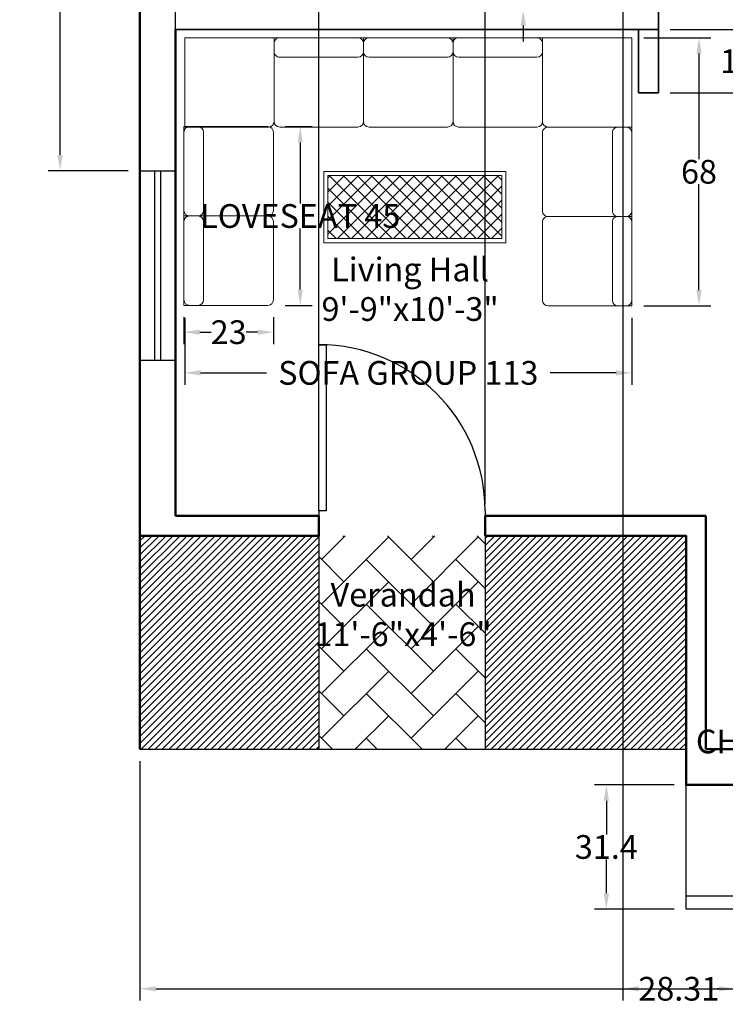
# Model space of a CAD drawing. Units: inches. Extents: x 89 to 490, y -59 to 378.
# Tile 1 of 20: x 97 to 275, y -51 to 198. Entities that reach past the tile are written whole.
import ezdxf

# ---------------------------------------------------------------- set-up
doc = ezdxf.new("R2010")
doc.units = ezdxf.units.IN
doc.header["$MEASUREMENT"] = 0
for name, color, linetype, lineweight in [('A-ANNO-DIMS', 2, 'Continuous', 18), ('A-AREA-IDEN', 7, 'Continuous', 18), ('A-FLOR-PATT', 3, 'Continuous', 13), ('A-FURN-PATT', 55, 'Continuous', 13), ('Center Table', 54, 'Continuous', 18), ('Doors', 34, 'Continuous', 25), ('Inner Walls', 31, 'Continuous', 35), ('L-PLNT-EDGE', 31, 'Continuous', 25), ('Outer Walls', 12, 'Continuous', 50), ('Sofa', 114, 'Continuous', 18), ('Verandah', 3, 'Continuous', 25), ('Windows', 171, 'Continuous', 25)]:
    doc.layers.add(name, color=color, linetype=linetype, lineweight=lineweight)
doc.styles.get("Standard").update_dxf_attribs({"font": 'arial.ttf'})
doc.dimstyles.get("Standard").update_dxf_attribs({"dimtxt": 6, "dimasz": 4, "dimexe": 3, "dimexo": 3, "dimgap": 0.09, "dimtad": 0, "dimtih": 1, "dimtoh": 1, "dimdec": 1, "dimzin": 0, "dimdsep": 46, "dimlunit": 3, "dimtxsty": 'Standard', "dimcen": 0.09, "dimadec": 0, "dimazin": 0, "dimtfac": 1, "dimtdec": 1, "dimtofl": 0, "dimtmove": 0, "dimatfit": 3, "dimfxl": 1, "dimtolj": 1, "dimtzin": 0, "dimarcsym": 0})

# ---------------------------------------------------------------- blocks, each defined once
blk = doc.blocks.new('*U6')
for p, q in [((0, 0), (0, -6)), ((40, 0), (40, -6))]:
    blk.add_line(p, q)
blk.add_lwpolyline([(0, 0), (0, 40), (1.75, 40), (1.75, 0)], close=True)
blk.add_arc((0, 0), 40, 0, 90)
blk = doc.blocks.new('A$C51FB459E')
for p, q in [((0, 1.6), (0, 2.4)), ((0, 2.4), (0.75, 2.4)), ((0.05, 2.4), (0.125, 2.4)), ((0, 1.65), (0, 2.35)), ((0.175, 2.35), (0.175, 1.65)), ((0.8, 2.35), (0.8, 1.65)), ((0, 0.8), (0, 1.6)), ((0, 1.6), (0.75, 1.6)), ((0.75, 1.6), (0, 1.6)), ((0.05, 1.6), (0.125, 1.6)), ((0.125, 1.6), (0.05, 1.6)), ((0, 0.85), (0, 1.55)), ((0.175, 1.55), (0.175, 0.85)), ((0.8, 1.55), (0.8, 0.85)), ((0, 0), (0, 0.8)), ((0, 0.8), (0.75, 0.8)), ((0.75, 0.8), (0, 0.8)), ((0.125, 0.8), (0.05, 0.8)), ((0.85, 0.8), (1.55, 0.8)), ((1.65, 0.8), (2.35, 0.8)), ((2.45, 0.8), (3.15, 0.8)), ((3.9996, 0.8), (3.25, 0.8)), ((3.9996, 0), (3.9996, 0.8)), ((0.8, 0), (0.8, 0.75)), ((0.8, 0.75), (0.8, 0)), ((1.6, 0), (1.6, 0.75)), ((1.6, 0.75), (1.6, 0)), ((2.4, 0.75), (2.4, 0)), ((2.4, 0), (2.4, 0.75)), ((3.2, 0.75), (3.2, 0)), ((3.2, 0.75), (3.2, 0)), ((0.8, 0.05), (0.8, 0.125)), ((0.85, 0.175), (1.55, 0.175)), ((1.6, 0.05), (1.6, 0.125)), ((1.6, 0.125), (1.6, 0.05)), ((1.65, 0.175), (2.35, 0.175)), ((2.4, 0.125), (2.4, 0.05)), ((2.4, 0.05), (2.4, 0.125)), ((2.45, 0.175), (3.15, 0.175)), ((3.2, 0.125), (3.2, 0.05)), ((0.8, 0), (0, 0)), ((1.6, 0), (0.8, 0)), ((1.55, 0), (0.85, 0)), ((2.4, 0), (1.6, 0)), ((2.35, 0), (1.65, 0)), ((3.2, 0), (2.4, 0)), ((3.15, 0), (2.45, 0)), ((3.2, 0), (3.9996, 0))]:
    blk.add_line(p, q)
for centre, start, end in [((0.05, 2.35), 90, 180), ((0.125, 2.35), 0, 90), ((0.75, 2.35), 0, 90), ((0.05, 1.65), 180, 270), ((0.05, 1.55), 90, 180), ((0.125, 1.65), 270, 0), ((0.125, 1.55), 360, 90), ((0.75, 1.65), 270, 0), ((0.75, 1.55), 360, 90), ((0.05, 0.85), 180, 270), ((0.125, 0.85), 270, 0), ((0.75, 0.85), 270, 0), ((0.75, 0.75), 0, 90), ((0.85, 0.75), 90, 180), ((1.55, 0.75), 0, 90), ((1.65, 0.75), 90, 180), ((2.35, 0.75), 0, 90), ((2.45, 0.75), 90, 180), ((3.15, 0.75), 0, 90), ((3.25, 0.75), 90, 180), ((0.85, 0.125), 90, 180), ((1.55, 0.125), 0, 90), ((1.65, 0.125), 90, 180), ((2.35, 0.125), 0, 90), ((2.45, 0.125), 90, 180), ((3.15, 0.125), 360, 90), ((0.85, 0.05), 180, 270), ((1.55, 0.05), 270, 0), ((1.65, 0.05), 180, 270), ((2.35, 0.05), 270, 360), ((2.45, 0.05), 180, 270), ((3.15, 0.05), 270, 0)]:
    blk.add_arc(centre, 0.05, start, end)
blk = doc.blocks.new('small sofa')
for p, q in [((881.35, 152.51), (860.16, 152.51)), ((860.16, 152.51), (881.35, 152.51)), ((877.82, 152.51), (879.94, 152.51)), ((881.35, 152.51), (881.35, 129.91)), ((858.75, 131.32), (858.75, 151.1)), ((876.41, 131.32), (876.41, 151.1)), ((881.35, 151.1), (881.35, 131.32)), ((881.35, 129.91), (860.16, 129.91)), ((860.16, 129.91), (881.35, 129.91)), ((879.94, 129.91), (877.82, 129.91)), ((877.82, 129.91), (879.94, 129.91)), ((881.35, 129.91), (881.35, 107.31)), ((858.75, 108.72), (858.75, 128.5)), ((876.41, 108.72), (876.41, 128.5)), ((881.35, 128.5), (881.35, 108.72)), ((881.35, 107.31), (860.16, 107.31)), ((879.94, 107.31), (877.82, 107.31))]:
    blk.add_line(p, q)
for centre, start, end in [((860.16, 151.1), 90, 180), ((877.82, 151.1), 90, 180), ((879.94, 151.1), 0, 90), ((860.16, 131.32), 180, 270), ((860.16, 128.5), 90, 180), ((877.82, 131.32), 180, 270), ((877.82, 128.5), 90, 180), ((879.94, 131.32), 270, 0), ((879.94, 128.5), 0, 90), ((860.16, 108.72), 180, 270), ((877.82, 108.72), 180, 270), ((879.94, 108.72), 270, 0)]:
    blk.add_arc(centre, 1.41, start, end)
blk = doc.blocks.new('WIN-48x9')
for p, q in [((3.8, 0), (3.8, 48)), ((5.2, 48), (5.2, 0))]:
    blk.add_line(p, q)
blk.add_lwpolyline([(9, 0), (0, 0), (0, 48), (9, 48)], close=True)
blk = doc.blocks.new('*D28')
at = {"layer": 'A-ANNO-DIMS', "color": 0, "lineweight": -2, "transparency": 16777216}
for p, q in [((326.43, 33.4), (324.38, 33.4)), ((327.38, 29.4), (327.38, 23.72)), ((326.43, 19.72), (324.38, 19.72)), ((327.38, 19.72), (327.38, 15.72)), ((327.38, 15.72), (323.38, 15.72))]:
    blk.add_line(p, q, dxfattribs=at)
at = {"layer": 'A-ANNO-DIMS', "color": 0, "transparency": 16777216}
for points in [[(326.71, 29.4), (328.05, 29.4), (327.38, 33.4)], [(326.71, 23.72), (328.05, 23.72), (327.38, 19.72)]]:
    blk.add_solid(points, dxfattribs=at)
at = {"layer": 'Defpoints', "color": 0, "transparency": 16777216}
for p in [(329.43, 33.4), (327.38, 19.72), (329.43, 19.72)]:
    blk.add_point(p, dxfattribs=at)
at = {"layer": 'A-ANNO-DIMS', "color": 0, "transparency": 16777216, "insert": (294.52, 15.72), "char_height": 6, "attachment_point": 5}
blk.add_mtext('\\A1;CHAIR 14 TYP.', dxfattribs=at)
blk = doc.blocks.new('*D38')
at = {"layer": 'A-ANNO-DIMS', "color": 0, "lineweight": -2, "transparency": 16777216}
for p, q in [((138.75, 122.88), (138.75, 105.93)), ((251.75, 122.88), (251.75, 105.93)), ((142.75, 108.93), (159.44, 108.93)), ((247.75, 108.93), (231.06, 108.93))]:
    blk.add_line(p, q, dxfattribs=at)
at = {"layer": 'A-ANNO-DIMS', "color": 0, "transparency": 16777216}
for points in [[(142.75, 109.59), (142.75, 108.26), (138.75, 108.93)], [(247.75, 109.59), (247.75, 108.26), (251.75, 108.93)]]:
    blk.add_solid(points, dxfattribs=at)
at = {"layer": 'Defpoints', "color": 0, "transparency": 16777216}
for p in [(138.75, 125.88), (251.75, 125.88), (138.75, 108.93)]:
    blk.add_point(p, dxfattribs=at)
at = {"layer": 'A-ANNO-DIMS', "color": 0, "transparency": 16777216, "insert": (195.25, 108.93), "char_height": 6, "attachment_point": 5}
blk.add_mtext('\\A1;SOFA GROUP 113', dxfattribs=at)
blk = doc.blocks.new('*D39')
at = {"layer": 'A-ANNO-DIMS', "color": 0, "lineweight": -2, "transparency": 16777216}
for p, q in [((254.75, 193.68), (271.7, 193.68)), ((268.7, 189.68), (268.7, 162.93)), ((268.7, 129.88), (268.7, 156.63)), ((254.75, 125.88), (271.7, 125.88))]:
    blk.add_line(p, q, dxfattribs=at)
at = {"layer": 'A-ANNO-DIMS', "color": 0, "transparency": 16777216}
for points in [[(268.04, 189.68), (269.37, 189.68), (268.7, 193.68)], [(268.04, 129.88), (269.37, 129.88), (268.7, 125.88)]]:
    blk.add_solid(points, dxfattribs=at)
at = {"layer": 'Defpoints', "color": 0, "transparency": 16777216}
for p in [(251.75, 193.68), (251.75, 125.88), (268.7, 125.88)]:
    blk.add_point(p, dxfattribs=at)
at = {"layer": 'A-ANNO-DIMS', "color": 0, "transparency": 16777216, "insert": (268.7, 159.78), "char_height": 6, "attachment_point": 5}
blk.add_mtext('\\A1;68', dxfattribs=at)
blk = doc.blocks.new('*D40')
at = {"layer": 'A-ANNO-DIMS', "color": 0, "lineweight": -2, "transparency": 16777216}
for p, q in [((164.17, 171.2), (170.95, 171.2)), ((167.95, 167.2), (167.95, 151.8)), ((167.95, 130), (167.95, 145.41)), ((164.17, 126), (170.95, 126))]:
    blk.add_line(p, q, dxfattribs=at)
at = {"layer": 'A-ANNO-DIMS', "color": 0, "transparency": 16777216}
for points in [[(167.29, 167.2), (168.62, 167.2), (167.95, 171.2)], [(167.29, 130), (168.62, 130), (167.95, 126)]]:
    blk.add_solid(points, dxfattribs=at)
at = {"layer": 'Defpoints', "color": 0, "transparency": 16777216}
for p in [(161.17, 171.2), (161.17, 126), (167.95, 126)]:
    blk.add_point(p, dxfattribs=at)
at = {"layer": 'A-ANNO-DIMS', "color": 0, "transparency": 16777216, "insert": (167.95, 148.6), "char_height": 6, "attachment_point": 5}
blk.add_mtext('\\A1;LOVESEAT 45', dxfattribs=at)
blk = doc.blocks.new('*D41')
at = {"layer": 'A-ANNO-DIMS', "color": 0, "lineweight": -2, "transparency": 16777216}
for p, q in [((138.57, 123), (138.57, 116.22)), ((161.17, 123), (161.17, 116.22)), ((142.57, 119.22), (145.43, 119.22)), ((157.17, 119.22), (154.31, 119.22))]:
    blk.add_line(p, q, dxfattribs=at)
at = {"layer": 'A-ANNO-DIMS', "color": 0, "transparency": 16777216}
for points in [[(142.57, 119.89), (142.57, 118.55), (138.57, 119.22)], [(157.17, 119.89), (157.17, 118.55), (161.17, 119.22)]]:
    blk.add_solid(points, dxfattribs=at)
at = {"layer": 'Defpoints', "color": 0, "transparency": 16777216}
for p in [(138.57, 126), (161.17, 126), (138.57, 119.22)]:
    blk.add_point(p, dxfattribs=at)
at = {"layer": 'A-ANNO-DIMS', "color": 0, "transparency": 16777216, "insert": (149.87, 119.22), "char_height": 6, "attachment_point": 5}
blk.add_mtext('\\A1;23', dxfattribs=at)
blk = doc.blocks.new('*D48')
at = {"layer": 'A-ANNO-DIMS', "color": 0, "lineweight": -2, "transparency": 16777216}
for p, q in [((127.44, 10.74), (127.44, -49.81)), ((459.44, -29.66), (459.44, -49.81)), ((131.44, -46.81), (286.76, -46.81)), ((455.44, -46.81), (300.13, -46.81))]:
    blk.add_line(p, q, dxfattribs=at)
at = {"layer": 'A-ANNO-DIMS', "color": 0, "transparency": 16777216}
for points in [[(131.44, -46.14), (131.44, -47.48), (127.44, -46.81)], [(455.44, -46.14), (455.44, -47.48), (459.44, -46.81)]]:
    blk.add_solid(points, dxfattribs=at)
at = {"layer": 'Defpoints', "color": 0, "transparency": 16777216}
for p in [(127.44, 13.74), (459.44, -26.66), (459.44, -46.81)]:
    blk.add_point(p, dxfattribs=at)
at = {"layer": 'A-ANNO-DIMS', "color": 0, "transparency": 16777216, "insert": (293.44, -46.81), "char_height": 6, "attachment_point": 5}
blk.add_mtext('\\A1;332', dxfattribs=at)
blk = doc.blocks.new('*D50')
at = {"layer": 'A-ANNO-DIMS', "color": 0, "lineweight": -2, "transparency": 16777216}
for p, q in [((262.44, 4.74), (242.29, 4.74)), ((245.29, 0.74), (245.29, -7.8)), ((245.29, -22.66), (245.29, -14.11)), ((262.44, -26.66), (242.29, -26.66))]:
    blk.add_line(p, q, dxfattribs=at)
at = {"layer": 'A-ANNO-DIMS', "color": 0, "transparency": 16777216}
for points in [[(244.62, 0.74), (245.96, 0.74), (245.29, 4.74)], [(244.62, -22.66), (245.96, -22.66), (245.29, -26.66)]]:
    blk.add_solid(points, dxfattribs=at)
at = {"layer": 'Defpoints', "color": 0, "transparency": 16777216}
for p in [(245.29, 4.74), (265.44, 4.74), (265.44, -26.66)]:
    blk.add_point(p, dxfattribs=at)
at = {"layer": 'A-ANNO-DIMS', "color": 0, "transparency": 16777216, "insert": (245.29, -10.96), "char_height": 6, "attachment_point": 5}
blk.add_mtext('\\A1;31.4', dxfattribs=at)
blk = doc.blocks.new('*D52')
at = {"layer": 'A-ANNO-DIMS', "color": 0, "lineweight": -2, "transparency": 16777216}
for p, q in [((124.44, 253.3), (104.29, 253.3)), ((107.29, 249.3), (107.29, 209.83)), ((107.29, 164.06), (107.29, 203.52)), ((124.44, 160.06), (104.29, 160.06))]:
    blk.add_line(p, q, dxfattribs=at)
at = {"layer": 'A-ANNO-DIMS', "color": 0, "transparency": 16777216}
for points in [[(106.62, 249.3), (107.96, 249.3), (107.29, 253.3)], [(106.62, 164.06), (107.96, 164.06), (107.29, 160.06)]]:
    blk.add_solid(points, dxfattribs=at)
at = {"layer": 'Defpoints', "color": 0, "transparency": 16777216}
for p in [(127.44, 253.3), (107.29, 160.06), (127.44, 160.06)]:
    blk.add_point(p, dxfattribs=at)
at = {"layer": 'A-ANNO-DIMS', "color": 0, "transparency": 16777216, "insert": (107.29, 206.68), "char_height": 6, "attachment_point": 5}
blk.add_mtext('\\A1;93.25', dxfattribs=at)
blk = doc.blocks.new('*D57')
at = {"layer": 'A-ANNO-DIMS', "color": 0, "lineweight": -2, "transparency": 16777216}
for p, q in [((172.65, 75.74), (172.65, 376.89)), ((214.65, 75.74), (214.65, 376.89)), ((176.65, 373.89), (189.17, 373.89)), ((210.65, 373.89), (198.13, 373.89))]:
    blk.add_line(p, q, dxfattribs=at)
at = {"layer": 'A-ANNO-DIMS', "color": 0, "transparency": 16777216}
for points in [[(176.65, 374.56), (176.65, 373.22), (172.65, 373.89)], [(210.65, 374.56), (210.65, 373.22), (214.65, 373.89)]]:
    blk.add_solid(points, dxfattribs=at)
at = {"layer": 'Defpoints', "color": 0, "transparency": 16777216}
for p in [(214.65, 373.89), (172.65, 72.74), (214.65, 72.74)]:
    blk.add_point(p, dxfattribs=at)
at = {"layer": 'A-ANNO-DIMS', "color": 0, "transparency": 16777216, "insert": (193.65, 373.89), "char_height": 6, "attachment_point": 5}
blk.add_mtext('\\A1;42', dxfattribs=at)
blk = doc.blocks.new('*D58')
at = {"layer": 'A-ANNO-DIMS', "color": 0, "lineweight": -2, "transparency": 16777216}
for p, q in [((136.44, 75.74), (136.44, 376.89)), ((172.65, 75.74), (172.65, 376.89)), ((140.44, 373.89), (142, 373.89)), ((168.65, 373.89), (167.08, 373.89))]:
    blk.add_line(p, q, dxfattribs=at)
at = {"layer": 'A-ANNO-DIMS', "color": 0, "transparency": 16777216}
for points in [[(140.44, 374.56), (140.44, 373.22), (136.44, 373.89)], [(168.65, 374.56), (168.65, 373.22), (172.65, 373.89)]]:
    blk.add_solid(points, dxfattribs=at)
at = {"layer": 'Defpoints', "color": 0, "transparency": 16777216}
for p in [(172.65, 373.89), (136.44, 72.74), (172.65, 72.74)]:
    blk.add_point(p, dxfattribs=at)
at = {"layer": 'A-ANNO-DIMS', "color": 0, "transparency": 16777216, "insert": (154.54, 373.89), "char_height": 6, "attachment_point": 5}
blk.add_mtext('\\A1;36.206', dxfattribs=at)
blk = doc.blocks.new('*D60')
at = {"layer": 'A-ANNO-DIMS', "color": 0, "lineweight": -2, "transparency": 16777216}
for p, q in [((224.29, 210.74), (224.29, 214.74)), ((224.29, 214.74), (228.29, 214.74)), ((241.44, 206.74), (221.29, 206.74)), ((241.44, 200.74), (221.29, 200.74)), ((224.29, 196.74), (224.29, 192.74))]:
    blk.add_line(p, q, dxfattribs=at)
at = {"layer": 'A-ANNO-DIMS', "color": 0, "transparency": 16777216}
for points in [[(223.62, 210.74), (224.96, 210.74), (224.29, 206.74)], [(223.62, 196.74), (224.96, 196.74), (224.29, 200.74)]]:
    blk.add_solid(points, dxfattribs=at)
at = {"layer": 'Defpoints', "color": 0, "transparency": 16777216}
for p in [(224.29, 206.74), (244.44, 206.74), (244.44, 200.74)]:
    blk.add_point(p, dxfattribs=at)
at = {"layer": 'A-ANNO-DIMS', "color": 0, "transparency": 16777216, "insert": (230.36, 214.74), "char_height": 6, "attachment_point": 5}
blk.add_mtext('\\A1;6', dxfattribs=at)
blk = doc.blocks.new('*D70')
at = {"layer": 'A-ANNO-DIMS', "color": 0, "lineweight": -2, "transparency": 16777216}
for p, q in [((261.44, 195.74), (281.59, 195.74)), ((278.59, 191.74), (278.59, 190.89)), ((278.59, 183.74), (278.59, 184.59)), ((261.44, 179.74), (281.59, 179.74))]:
    blk.add_line(p, q, dxfattribs=at)
at = {"layer": 'A-ANNO-DIMS', "color": 0, "transparency": 16777216}
for points in [[(277.92, 191.74), (279.26, 191.74), (278.59, 195.74)], [(277.92, 183.74), (279.26, 183.74), (278.59, 179.74)]]:
    blk.add_solid(points, dxfattribs=at)
at = {"layer": 'Defpoints', "color": 0, "transparency": 16777216}
for p in [(258.44, 195.74), (258.44, 179.74), (278.59, 179.74)]:
    blk.add_point(p, dxfattribs=at)
at = {"layer": 'A-ANNO-DIMS', "color": 0, "transparency": 16777216, "insert": (278.59, 187.74), "char_height": 6, "attachment_point": 5}
blk.add_mtext('\\A1;16', dxfattribs=at)
blk = doc.blocks.new('*D74')
at = {"layer": 'A-ANNO-DIMS', "color": 0, "lineweight": -2, "transparency": 16777216}
for p, q in [((249.44, 341.74), (249.44, -49.81)), ((277.75, 341.35), (277.75, -49.81)), ((253.44, -46.81), (253.91, -46.81)), ((273.75, -46.81), (273.28, -46.81))]:
    blk.add_line(p, q, dxfattribs=at)
at = {"layer": 'A-ANNO-DIMS', "color": 0, "transparency": 16777216}
for points in [[(253.44, -46.14), (253.44, -47.48), (249.44, -46.81)], [(273.75, -46.14), (273.75, -47.48), (277.75, -46.81)]]:
    blk.add_solid(points, dxfattribs=at)
at = {"layer": 'Defpoints', "color": 0, "transparency": 16777216}
for p in [(249.44, 344.74), (277.75, 344.35), (277.75, -46.81)]:
    blk.add_point(p, dxfattribs=at)
at = {"layer": 'A-ANNO-DIMS', "color": 0, "transparency": 16777216, "insert": (263.6, -46.81), "char_height": 6, "attachment_point": 5}
blk.add_mtext('\\A1;28.31', dxfattribs=at)

msp = doc.modelspace()

# ---------------------------------------------------------------- hatches: boundary and pattern name
at = {"layer": 'A-FLOR-PATT'}
h = msp.add_hatch(dxfattribs=at)
h.set_pattern_fill('ANSI31', color=256, scale=10)
h.set_pattern_definition([(45, (-188.7147, -85.3119), (-0.8838835, 0.8838835), [])])
h.paths.add_polyline_path([(265.4414, 67.7413), (214.6478, 67.7413), (214.6478, 13.7413), (265.4414, 13.7413)])
h.paths.add_polyline_path([(172.6478, 67.7413), (127.4414, 67.7413), (127.4414, 13.7413), (172.6478, 13.7413)])
h = msp.add_hatch(dxfattribs=at)
h.set_pattern_fill('AR-HBONE', color=256, scale=2)
h.set_pattern_definition([(45, (-188.715, -85.312), (0, 11.31371), [24, -8]), (135, (-183.058, -79.655), (9e-16, 11.31371), [24, -8])])
h.paths.add_polyline_path([(214.6478, 67.7413), (172.6478, 67.7413), (172.6478, 13.7413), (214.6478, 13.7413)])
at = {"layer": 'A-FURN-PATT'}
h = msp.add_hatch(dxfattribs=at)
h.set_pattern_fill('ANSI37', color=256, scale=20)
h.set_pattern_definition([(45, (-188.7147, -85.312), (-1.767767, 1.767767), []), (135, (-188.7147, -85.312), (-1.767767, -1.767767), [])])
h.paths.add_polyline_path([(218.8877, 158.8206), (174.9559, 158.8206), (174.9559, 142.8888), (218.8877, 142.8888)])

# ---------------------------------------------------------------- linework, layer by layer
at = {"layer": 'Center Table'}
for points in [[(173.9218, 159.8547), (219.9218, 159.8547), (219.9218, 141.8547), (173.9218, 141.8547)], [(174.9559, 158.8206), (218.8877, 158.8206), (218.8877, 142.8888), (174.9559, 142.8888)]]:
    msp.add_lwpolyline(points, close=True, dxfattribs=at)
at = {"layer": 'Inner Walls'}
for p, q in [((258.4414, 195.7413), (258.4414, 200.7413)), ((136.4414, 195.7413), (258.4414, 195.7413)), ((253.4414, 195.7413), (253.4414, 179.7413)), ((258.4414, 195.7413), (258.4414, 179.7413)), ((258.4414, 179.7413), (253.4414, 179.7413))]:
    msp.add_line(p, q, dxfattribs=at)
at = {"layer": 'L-PLNT-EDGE'}
for p, q in [((265.4414, -26.6594), (265.4414, 4.7413)), ((459.4414, -23.3886), (265.4414, -23.3886)), ((459.4414, -26.6594), (265.4414, -26.6594))]:
    msp.add_line(p, q, dxfattribs=at)
at = {"layer": 'Outer Walls'}
for p, q in [((136.4414, 72.7413), (136.4414, 195.7413)), ((136.4414, 72.7413), (172.6478, 72.7413)), ((172.6478, 67.7413), (172.6478, 72.7413)), ((214.6478, 67.7413), (214.6478, 72.7413)), ((214.6478, 72.7413), (270.4414, 72.7413)), ((270.4414, 13.7413), (270.4414, 72.7413)), ((127.4414, 67.7413), (172.6478, 67.7413)), ((270.4414, 13.7413), (450.4414, 13.7413))]:
    msp.add_line(p, q, dxfattribs=at)
msp.add_lwpolyline([(214.6478, 67.7413), (265.4414, 67.7413), (265.4414, 4.7413), (459.4414, 4.7413), (459.4414, 353.7413), (127.4414, 353.7413), (127.4414, 13.7413)], dxfattribs=at)
at = {"layer": 'Verandah'}
for p, q in [((172.6478, 67.7413), (172.6478, 13.7413)), ((214.6478, 67.7413), (214.6478, 13.7413)), ((127.4414, 13.7413), (265.4414, 13.7413))]:
    msp.add_line(p, q, dxfattribs=at)

# ---------------------------------------------------------------- block references
at = {"layer": 'Doors', "xscale": 1.05, "yscale": 1.05, "zscale": 1.05}
msp.add_blockref('*U6', (172.6478, 74.0413), dxfattribs=at)
at = {"layer": 'Sofa', "xscale": 28.25282528252755, "yscale": 28.25282528252755, "zscale": 28.25282528252755, "rotation": 180}
msp.add_blockref('A$C51FB459E', (251.7525, 193.6826), dxfattribs=at)
at = {"layer": 'Sofa', "rotation": 180}
msp.add_blockref('small sofa', (1019.9262, 278.5098), dxfattribs=at)
at = {"layer": 'Windows'}
msp.add_blockref('WIN-48x9', (127.441, 112.055), dxfattribs=at)

# ---------------------------------------------------------------- texts
at = {"layer": 'A-AREA-IDEN', "char_height": 6, "attachment_point": 1}
for s, insert in [('\\pxqc;Living Hall\\P9\'-9"x10\'-3"', (172.5056, 138.0781)), ('\\pxqc;Verandah\\P11\'-6"x4\'-6"', (170.7306, 55.8341))]:
    msp.add_mtext_dynamic_manual_height_columns(s, width=46.403971, gutter_width=1, heights=[0], dxfattribs=dict(at, insert=insert))

# ---------------------------------------------------------------- dimensions: what is measured, and where the dimension line sits
at = {"layer": 'A-ANNO-DIMS'}
for base, p1, p2, override, picture, middle in [((172.6478, 373.8913), (136.4414, 72.7413), (172.6478, 72.7413), {"dimdec": 3, "dimlfac": 1, "dimrnd": 0, "dimzin": 0, "dimdsep": 46, "dimlunit": 2}, '*D58', (154.5446, 373.8913)), ((214.6478, 373.8913), (172.6478, 72.7413), (214.6478, 72.7413), {"dimdec": 0, "dimlfac": 1, "dimrnd": 0, "dimzin": 0, "dimdsep": 46, "dimlunit": 2}, '*D57', (193.6478, 373.8913)), ((277.7535, -46.8094), (249.4414, 344.7413), (277.7535, 344.3468), {"dimdec": 2, "dimlfac": 1, "dimrnd": 0, "dimzin": 0, "dimdsep": 46, "dimlunit": 2}, '*D74', (263.5974, -46.8094)), ((459.4414, -46.8094), (127.4414, 13.7413), (459.4414, -26.6594), {"dimdec": 0, "dimlfac": 1, "dimrnd": 0, "dimzin": 0, "dimdsep": 46, "dimlunit": 2}, '*D48', (293.4414, -46.8094))]:
    dim = msp.add_linear_dim(base=base, p1=p1, p2=p2, dimstyle='Standard', override=override, dxfattribs=at)
    dim.commit()
    dim.dimension.update_dxf_attribs({"geometry": picture, "text_midpoint": middle})
for base, p1, p2, angle, override, picture, middle in [((107.2914, 160.055), (127.4414, 253.3003), (127.4414, 160.055), 90, {"dimdec": 2, "dimlfac": 1, "dimrnd": 0, "dimzin": 0, "dimdsep": 46, "dimlunit": 2}, '*D52', (107.2914, 206.6776)), ((224.2914, 206.7413), (244.4414, 200.7413), (244.4414, 206.7413), 90, {"dimdec": 0, "dimlfac": 1, "dimrnd": 0, "dimzin": 0, "dimdsep": 46, "dimlunit": 2}, '*D60', (230.3623, 214.7413)), ((278.5914, 179.7413), (258.4414, 195.7413), (258.4414, 179.7413), 270, {"dimdec": 0, "dimlfac": 1, "dimrnd": 0, "dimzin": 0, "dimdsep": 46, "dimlunit": 2}, '*D70', (278.5914, 187.7413)), ((268.7025, 125.8758), (251.7525, 193.6826), (251.7525, 125.8758), 270, {"dimdec": 0, "dimlfac": 1, "dimrnd": 0, "dimzin": 0, "dimdsep": 46, "dimlunit": 2}, '*D39', (268.7025, 159.7792)), ((138.5715, 119.2184), (161.1738, 125.9991), (138.5715, 125.9991), 180, {"dimdec": 0, "dimlfac": 1, "dimrnd": 0, "dimzin": 0, "dimdsep": 46, "dimlunit": 2}, '*D41', (149.8727, 119.2184)), ((245.2914, 4.7413), (265.4414, -26.6594), (265.4414, 4.7413), 90, {"dimdec": 1, "dimlfac": 1, "dimrnd": 0, "dimzin": 0, "dimdsep": 46, "dimlunit": 2}, '*D50', (245.2914, -10.9591))]:
    dim = msp.add_linear_dim(base=base, p1=p1, p2=p2, angle=angle, dimstyle='Standard', override=override, dxfattribs=at)
    dim.commit()
    dim.dimension.update_dxf_attribs({"geometry": picture, "text_midpoint": middle})
for base, p1, p2, angle, text, picture, middle in [((167.9545, 125.9991), (161.1738, 171.2036), (161.1738, 125.9991), 270, 'LOVESEAT <>', '*D40', (167.9545, 148.6013)), ((138.7525, 108.9258), (251.7525, 125.8758), (138.7525, 125.8758), 180, 'SOFA GROUP <>', '*D38', (195.2525, 108.9258)), ((327.3791, 19.7198), (329.4308, 33.3978), (329.4308, 19.7198), 270, 'CHAIR <> TYP.', '*D28', (294.517, 15.7198))]:
    dim = msp.add_linear_dim(base=base, p1=p1, p2=p2, angle=angle, text=text, dimstyle='Standard', override={"dimdec": 0, "dimlfac": 1, "dimrnd": 0, "dimzin": 0, "dimdsep": 46, "dimlunit": 2}, dxfattribs=at)
    dim.commit()
    dim.dimension.update_dxf_attribs({"geometry": picture, "text_midpoint": middle})

doc.saveas('drawing.dxf')
